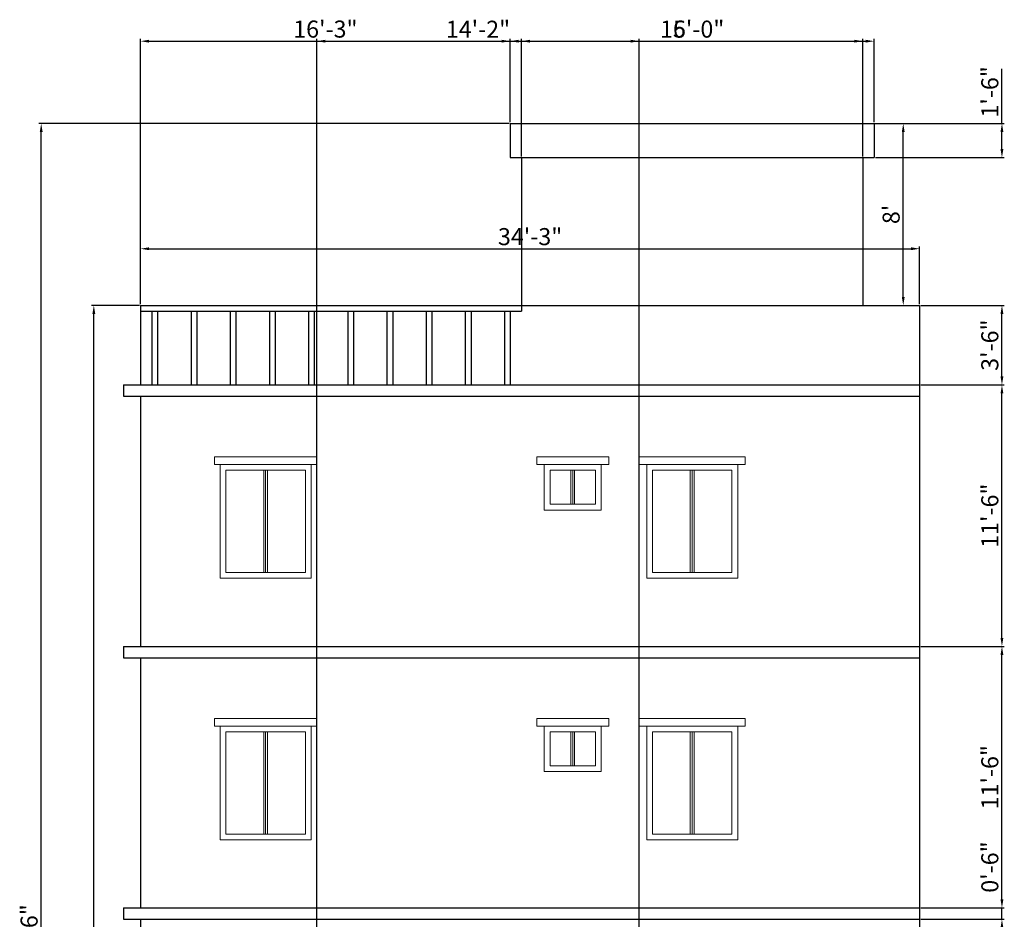
# Model space of a CAD drawing. Units: inches. Extents: x 1692 to 2762, y 798 to 1757.
# Tile 2 of 4: x 1692 to 2211, y 1282 to 1757. Entities that reach past the tile are written whole.
import ezdxf

# ---------------------------------------------------------------- set-up
doc = ezdxf.new("R2010")
doc.units = ezdxf.units.IN
for name, color, linetype, lineweight in [('A-ANNO-DIMS', 2, 'Continuous', 18), ('A-ELEV', 7, 'Continuous', 25), ('A-GLAZ', 4, 'Continuous', 18)]:
    doc.layers.add(name, color=color, linetype=linetype, lineweight=lineweight)
doc.styles.get("Standard").update_dxf_attribs({"font": 'arial.ttf'})
doc.dimstyles.new('ISO-25', dxfattribs={"dimtxt": 9, "dimasz": 4.5, "dimexe": 1.25, "dimexo": 0.625, "dimtad": 1, "dimdec": 0, "dimlunit": 3, "dimtxsty": 'Standard', "dimcen": 2.5, "dimadec": 0, "dimazin": 0, "dimtfac": 1, "dimtdec": 0, "dimtmove": 0, "dimatfit": 3, "dimfxl": 1, "dimarcsym": 0})

# ---------------------------------------------------------------- blocks, each defined once
blk = doc.blocks.new('*D12')
at = {"layer": 'A-ANNO-DIMS', "color": 0, "lineweight": -2, "transparency": 16777216}
for p, q in [((1755.16, 1606.43), (1729.9, 1606.43)), ((1731.15, 848.93), (1731.15, 1601.93)), ((1755.16, 844.43), (1729.9, 844.43))]:
    blk.add_line(p, q, dxfattribs=at)
at = {"layer": 'A-ANNO-DIMS', "color": 0, "lineweight": 0, "transparency": 16777216}
for points in [[(1730.4, 1601.93), (1731.9, 1601.93), (1731.15, 1606.43)], [(1730.4, 848.93), (1731.9, 848.93), (1731.15, 844.43)]]:
    blk.add_solid(points, dxfattribs=at)
at = {"layer": 'Defpoints', "color": 0, "lineweight": 0, "transparency": 16777216}
for p in [(1731.15, 1606.43), (1755.78, 1606.43), (1755.78, 844.43)]:
    blk.add_point(p, dxfattribs=at)
at = {"layer": 'A-ANNO-DIMS', "color": 0, "transparency": 16777216, "insert": (1725.92, 1225.43), "char_height": 9, "attachment_point": 5, "rotation": 90}
blk.add_mtext('63\'-6"', dxfattribs=at)
blk = doc.blocks.new('*D13')
at = {"layer": 'A-ANNO-DIMS', "color": 0, "lineweight": -2, "transparency": 16777216}
for p, q in [((1755.78, 1607.06), (1755.78, 1637.56)), ((1760.28, 1636.31), (2162.28, 1636.31)), ((2166.78, 1607.06), (2166.78, 1637.56))]:
    blk.add_line(p, q, dxfattribs=at)
at = {"layer": 'A-ANNO-DIMS', "color": 0, "lineweight": 0, "transparency": 16777216}
for points in [[(1760.28, 1637.06), (1760.28, 1635.56), (1755.78, 1636.31)], [(2162.28, 1637.06), (2162.28, 1635.56), (2166.78, 1636.31)]]:
    blk.add_solid(points, dxfattribs=at)
at = {"layer": 'Defpoints', "color": 0, "lineweight": 0, "transparency": 16777216}
for p in [(2166.78, 1636.31), (1755.78, 1606.43), (2166.78, 1606.43)]:
    blk.add_point(p, dxfattribs=at)
at = {"layer": 'A-ANNO-DIMS', "color": 0, "transparency": 16777216, "insert": (1961.28, 1641.54), "char_height": 9, "attachment_point": 5}
blk.add_mtext('34\'-3"', dxfattribs=at)
blk = doc.blocks.new('*D14')
at = {"layer": 'A-ANNO-DIMS', "color": 0, "lineweight": -2, "transparency": 16777216}
for p, q in [((2137.41, 1702.43), (2159.37, 1702.43)), ((2158.12, 1610.93), (2158.12, 1697.93)), ((2137.41, 1606.43), (2159.37, 1606.43))]:
    blk.add_line(p, q, dxfattribs=at)
at = {"layer": 'A-ANNO-DIMS', "color": 0, "lineweight": 0, "transparency": 16777216}
for points in [[(2157.37, 1697.93), (2158.87, 1697.93), (2158.12, 1702.43)], [(2157.37, 1610.93), (2158.87, 1610.93), (2158.12, 1606.43)]]:
    blk.add_solid(points, dxfattribs=at)
at = {"layer": 'Defpoints', "color": 0, "lineweight": 0, "transparency": 16777216}
for p in [(2136.78, 1702.43), (2158.12, 1702.43), (2136.78, 1606.43)]:
    blk.add_point(p, dxfattribs=at)
at = {"layer": 'A-ANNO-DIMS', "color": 0, "transparency": 16777216, "insert": (2152.9, 1654.43), "char_height": 9, "attachment_point": 5, "rotation": 90}
blk.add_mtext("8'", dxfattribs=at)
blk = doc.blocks.new('WIN-ELEV-L')
for p, q in [((1794.78, 974.43), (1848.78, 974.43)), ((1794.78, 974.43), (1794.78, 970.43)), ((1797.78, 974.43), (1794.78, 974.43)), ((1845.78, 974.43), (1848.78, 974.43)), ((1848.78, 974.43), (1848.78, 970.43)), ((1794.78, 970.43), (1848.78, 970.43)), ((1797.78, 970.43), (1797.78, 910.43)), ((1800.78, 967.43), (1842.78, 967.43)), ((1800.78, 967.43), (1800.78, 913.43)), ((1820.78, 967.43), (1820.78, 913.43)), ((1821.78, 967.43), (1821.78, 913.43)), ((1822.78, 967.43), (1822.78, 913.43)), ((1842.78, 967.43), (1842.78, 913.43)), ((1845.78, 970.43), (1845.78, 910.43)), ((1797.78, 910.43), (1845.78, 910.43)), ((1797.78, 910.43), (1845.78, 910.43)), ((1800.78, 913.43), (1842.78, 913.43))]:
    blk.add_line(p, q)
blk = doc.blocks.new('WIN-ELEV-R')
for p, q in [((2018.78, 1112.43), (2074.78, 1112.43)), ((2018.78, 1112.43), (2018.78, 1108.43)), ((2074.78, 1112.43), (2074.78, 1108.43)), ((2018.78, 1108.43), (2074.78, 1108.43)), ((2022.78, 1108.43), (2022.78, 1048.43)), ((2070.78, 1108.43), (2070.78, 1048.43)), ((2025.78, 1105.43), (2067.78, 1105.43)), ((2025.78, 1105.43), (2025.78, 1051.43)), ((2045.78, 1105.43), (2045.78, 1051.43)), ((2046.78, 1105.43), (2046.78, 1051.43)), ((2047.78, 1105.43), (2047.78, 1051.43)), ((2067.78, 1105.43), (2067.78, 1051.43)), ((2025.78, 1051.43), (2067.78, 1051.43)), ((2022.78, 1048.43), (2070.78, 1048.43))]:
    blk.add_line(p, q)
blk = doc.blocks.new('WIN-ELEV-S')
for p, q in [((1964.78, 974.43), (2002.78, 974.43)), ((1964.78, 974.43), (1964.78, 970.43)), ((2002.78, 974.43), (2002.78, 970.43)), ((1964.78, 970.43), (2002.78, 970.43)), ((1968.78, 970.43), (1968.78, 946.43)), ((1971.78, 967.43), (1995.78, 967.43)), ((1971.78, 967.43), (1971.78, 949.43)), ((1982.78, 967.43), (1982.78, 949.43)), ((1983.78, 967.43), (1983.78, 949.43)), ((1984.78, 967.43), (1984.78, 949.43)), ((1995.78, 967.43), (1995.78, 949.43)), ((1998.78, 970.43), (1998.78, 946.43)), ((1968.78, 946.43), (1998.78, 946.43)), ((1971.78, 949.43), (1995.78, 949.43))]:
    blk.add_line(p, q)
blk = doc.blocks.new('*D24')
at = {"layer": 'A-ANNO-DIMS', "color": 0, "lineweight": -2, "transparency": 16777216}
for p, q in [((1950.16, 1702.43), (1702.13, 1702.43)), ((1703.38, 848.93), (1703.38, 1697.93)), ((1746.16, 844.43), (1702.13, 844.43))]:
    blk.add_line(p, q, dxfattribs=at)
at = {"layer": 'A-ANNO-DIMS', "color": 0, "lineweight": 0, "transparency": 16777216}
for points in [[(1702.63, 1697.93), (1704.13, 1697.93), (1703.38, 1702.43)], [(1702.63, 848.93), (1704.13, 848.93), (1703.38, 844.43)]]:
    blk.add_solid(points, dxfattribs=at)
at = {"layer": 'Defpoints', "color": 0, "lineweight": 0, "transparency": 16777216}
for p in [(1703.38, 1702.43), (1950.78, 1702.43), (1746.78, 844.43)]:
    blk.add_point(p, dxfattribs=at)
at = {"layer": 'A-ANNO-DIMS', "color": 0, "transparency": 16777216, "insert": (1698.16, 1273.43), "char_height": 9, "attachment_point": 5, "rotation": 90}
blk.add_mtext('71\'-6"', dxfattribs=at)
blk = doc.blocks.new('*D34')
at = {"layer": 'A-ANNO-DIMS', "color": 0, "lineweight": -2, "transparency": 16777216}
for p, q in [((2210.18, 1292.93), (2210.18, 1322.61)), ((2167.41, 1288.43), (2211.43, 1288.43)), ((2210.18, 1282.43), (2210.18, 1288.43)), ((2167.41, 1282.43), (2211.43, 1282.43)), ((2210.18, 1277.93), (2210.18, 1273.43))]:
    blk.add_line(p, q, dxfattribs=at)
at = {"layer": 'A-ANNO-DIMS', "color": 0, "lineweight": 0, "transparency": 16777216}
for points in [[(2209.43, 1292.93), (2210.93, 1292.93), (2210.18, 1288.43)], [(2209.43, 1277.93), (2210.93, 1277.93), (2210.18, 1282.43)]]:
    blk.add_solid(points, dxfattribs=at)
at = {"layer": 'Defpoints', "color": 0, "lineweight": 0, "transparency": 16777216}
for p in [(2166.78, 1288.43), (2210.18, 1288.43), (2166.78, 1282.43)]:
    blk.add_point(p, dxfattribs=at)
at = {"layer": 'A-ANNO-DIMS', "color": 0, "transparency": 16777216, "insert": (2204.96, 1310.02), "char_height": 9, "attachment_point": 5, "rotation": 90}
blk.add_mtext('0\'-6"', dxfattribs=at)
blk = doc.blocks.new('*D35')
at = {"layer": 'A-ANNO-DIMS', "color": 0, "lineweight": -2, "transparency": 16777216}
for p, q in [((2167.41, 1426.43), (2211.43, 1426.43)), ((2210.18, 1292.93), (2210.18, 1421.93)), ((2167.41, 1288.43), (2211.43, 1288.43))]:
    blk.add_line(p, q, dxfattribs=at)
at = {"layer": 'A-ANNO-DIMS', "color": 0, "lineweight": 0, "transparency": 16777216}
for points in [[(2209.43, 1421.93), (2210.93, 1421.93), (2210.18, 1426.43)], [(2209.43, 1292.93), (2210.93, 1292.93), (2210.18, 1288.43)]]:
    blk.add_solid(points, dxfattribs=at)
at = {"layer": 'Defpoints', "color": 0, "lineweight": 0, "transparency": 16777216}
for p in [(2166.78, 1426.43), (2210.18, 1426.43), (2166.78, 1288.43)]:
    blk.add_point(p, dxfattribs=at)
at = {"layer": 'A-ANNO-DIMS', "color": 0, "transparency": 16777216, "insert": (2204.96, 1357.43), "char_height": 9, "attachment_point": 5, "rotation": 90}
blk.add_mtext('11\'-6"', dxfattribs=at)
blk = doc.blocks.new('*D36')
at = {"layer": 'A-ANNO-DIMS', "color": 0, "lineweight": -2, "transparency": 16777216}
for p, q in [((2167.41, 1564.43), (2211.43, 1564.43)), ((2210.18, 1430.93), (2210.18, 1559.93)), ((2167.41, 1426.43), (2211.43, 1426.43))]:
    blk.add_line(p, q, dxfattribs=at)
at = {"layer": 'A-ANNO-DIMS', "color": 0, "lineweight": 0, "transparency": 16777216}
for points in [[(2209.43, 1559.93), (2210.93, 1559.93), (2210.18, 1564.43)], [(2209.43, 1430.93), (2210.93, 1430.93), (2210.18, 1426.43)]]:
    blk.add_solid(points, dxfattribs=at)
at = {"layer": 'Defpoints', "color": 0, "lineweight": 0, "transparency": 16777216}
for p in [(2166.78, 1564.43), (2210.18, 1564.43), (2166.78, 1426.43)]:
    blk.add_point(p, dxfattribs=at)
at = {"layer": 'A-ANNO-DIMS', "color": 0, "transparency": 16777216, "insert": (2204.96, 1495.43), "char_height": 9, "attachment_point": 5, "rotation": 90}
blk.add_mtext('11\'-6"', dxfattribs=at)
blk = doc.blocks.new('*D37')
at = {"layer": 'A-ANNO-DIMS', "color": 0, "lineweight": -2, "transparency": 16777216}
for p, q in [((2167.41, 1606.43), (2211.43, 1606.43)), ((2210.18, 1568.93), (2210.18, 1601.93)), ((2167.41, 1564.43), (2211.43, 1564.43))]:
    blk.add_line(p, q, dxfattribs=at)
at = {"layer": 'A-ANNO-DIMS', "color": 0, "lineweight": 0, "transparency": 16777216}
for points in [[(2209.43, 1601.93), (2210.93, 1601.93), (2210.18, 1606.43)], [(2209.43, 1568.93), (2210.93, 1568.93), (2210.18, 1564.43)]]:
    blk.add_solid(points, dxfattribs=at)
at = {"layer": 'Defpoints', "color": 0, "lineweight": 0, "transparency": 16777216}
for p in [(2166.78, 1606.43), (2210.18, 1606.43), (2166.78, 1564.43)]:
    blk.add_point(p, dxfattribs=at)
at = {"layer": 'A-ANNO-DIMS', "color": 0, "transparency": 16777216, "insert": (2204.96, 1585.43), "char_height": 9, "attachment_point": 5, "rotation": 90}
blk.add_mtext('3\'-6"', dxfattribs=at)
blk = doc.blocks.new('*D38')
at = {"layer": 'A-ANNO-DIMS', "color": 0, "lineweight": -2, "transparency": 16777216}
for p, q in [((2210.18, 1702.43), (2210.18, 1731.26)), ((2143.41, 1702.43), (2211.43, 1702.43)), ((2210.18, 1688.93), (2210.18, 1697.93)), ((2143.41, 1684.43), (2211.43, 1684.43))]:
    blk.add_line(p, q, dxfattribs=at)
at = {"layer": 'A-ANNO-DIMS', "color": 0, "lineweight": 0, "transparency": 16777216}
for points in [[(2209.43, 1697.93), (2210.93, 1697.93), (2210.18, 1702.43)], [(2209.43, 1688.93), (2210.93, 1688.93), (2210.18, 1684.43)]]:
    blk.add_solid(points, dxfattribs=at)
at = {"layer": 'Defpoints', "color": 0, "lineweight": 0, "transparency": 16777216}
for p in [(2142.78, 1702.43), (2210.18, 1702.43), (2142.78, 1684.43)]:
    blk.add_point(p, dxfattribs=at)
at = {"layer": 'A-ANNO-DIMS', "color": 0, "transparency": 16777216, "insert": (2204.96, 1719.1), "char_height": 9, "attachment_point": 5, "rotation": 90}
blk.add_mtext('1\'-6"', dxfattribs=at)
blk = doc.blocks.new('*D47')
at = {"layer": 'A-ANNO-DIMS', "color": 0, "lineweight": -2, "transparency": 16777216}
for p, q in [((1848.78, 1113.06), (1848.78, 1747.08)), ((1853.28, 1745.83), (2014.28, 1745.83)), ((2018.78, 1113.06), (2018.78, 1747.08))]:
    blk.add_line(p, q, dxfattribs=at)
at = {"layer": 'A-ANNO-DIMS', "color": 0, "lineweight": 0, "transparency": 16777216}
for points in [[(1853.28, 1746.58), (1853.28, 1745.08), (1848.78, 1745.83)], [(2014.28, 1746.58), (2014.28, 1745.08), (2018.78, 1745.83)]]:
    blk.add_solid(points, dxfattribs=at)
at = {"layer": 'Defpoints', "color": 0, "lineweight": 0, "transparency": 16777216}
for p in [(2018.78, 1745.83), (1848.78, 1112.43), (2018.78, 1112.43)]:
    blk.add_point(p, dxfattribs=at)
at = {"layer": 'A-ANNO-DIMS', "color": 0, "transparency": 16777216, "insert": (1933.78, 1750.98), "char_height": 9, "attachment_point": 5}
blk.add_mtext('14\'-2"', dxfattribs=at)
blk = doc.blocks.new('*D48')
at = {"layer": 'A-ANNO-DIMS', "color": 0, "lineweight": -2, "transparency": 16777216}
for p, q in [((1755.78, 1607.06), (1755.78, 1747.08)), ((1760.28, 1745.83), (1946.28, 1745.83)), ((1950.78, 1703.06), (1950.78, 1747.08))]:
    blk.add_line(p, q, dxfattribs=at)
at = {"layer": 'A-ANNO-DIMS', "color": 0, "lineweight": 0, "transparency": 16777216}
for points in [[(1760.28, 1746.58), (1760.28, 1745.08), (1755.78, 1745.83)], [(1946.28, 1746.58), (1946.28, 1745.08), (1950.78, 1745.83)]]:
    blk.add_solid(points, dxfattribs=at)
at = {"layer": 'Defpoints', "color": 0, "lineweight": 0, "transparency": 16777216}
for p in [(1950.78, 1745.83), (1950.78, 1702.43), (1755.78, 1606.43)]:
    blk.add_point(p, dxfattribs=at)
at = {"layer": 'A-ANNO-DIMS', "color": 0, "transparency": 16777216, "insert": (1853.28, 1751.06), "char_height": 9, "attachment_point": 5}
blk.add_mtext('16\'-3"', dxfattribs=at)
blk = doc.blocks.new('*D49')
at = {"layer": 'A-ANNO-DIMS', "color": 0, "lineweight": -2, "transparency": 16777216}
for p, q in [((1950.78, 1703.06), (1950.78, 1747.08)), ((1955.28, 1745.83), (2138.28, 1745.83)), ((2142.78, 1703.06), (2142.78, 1747.08))]:
    blk.add_line(p, q, dxfattribs=at)
at = {"layer": 'A-ANNO-DIMS', "color": 0, "lineweight": 0, "transparency": 16777216}
for points in [[(1955.28, 1746.58), (1955.28, 1745.08), (1950.78, 1745.83)], [(2138.28, 1746.58), (2138.28, 1745.08), (2142.78, 1745.83)]]:
    blk.add_solid(points, dxfattribs=at)
at = {"layer": 'Defpoints', "color": 0, "lineweight": 0, "transparency": 16777216}
for p in [(2142.78, 1745.83), (1950.78, 1702.43), (2142.78, 1702.43)]:
    blk.add_point(p, dxfattribs=at)
at = {"layer": 'A-ANNO-DIMS', "color": 0, "transparency": 16777216, "insert": (2046.78, 1751.05), "char_height": 9, "attachment_point": 5}
blk.add_mtext('16\'-0"', dxfattribs=at)
blk = doc.blocks.new('*D50')
at = {"layer": 'A-ANNO-DIMS', "color": 0, "lineweight": -2, "transparency": 16777216}
for p, q in [((1956.78, 1685.06), (1956.78, 1747.08)), ((1961.28, 1745.83), (2132.28, 1745.83)), ((2136.78, 1685.06), (2136.78, 1747.08))]:
    blk.add_line(p, q, dxfattribs=at)
at = {"layer": 'A-ANNO-DIMS', "color": 0, "lineweight": 0, "transparency": 16777216}
for points in [[(1961.28, 1746.58), (1961.28, 1745.08), (1956.78, 1745.83)], [(2132.28, 1746.58), (2132.28, 1745.08), (2136.78, 1745.83)]]:
    blk.add_solid(points, dxfattribs=at)
at = {"layer": 'Defpoints', "color": 0, "lineweight": 0, "transparency": 16777216}
for p in [(2136.78, 1745.83), (1956.78, 1684.43), (2136.78, 1684.43)]:
    blk.add_point(p, dxfattribs=at)
at = {"layer": 'A-ANNO-DIMS', "color": 0, "transparency": 16777216, "insert": (2046.78, 1751.05), "char_height": 9, "attachment_point": 5}
blk.add_mtext('15\'-0"', dxfattribs=at)

msp = doc.modelspace()

# ---------------------------------------------------------------- linework, layer by layer
at = {"layer": 'A-ELEV'}
for p, q in [((1950.78, 1702.43), (2142.78, 1702.43)), ((1950.78, 1702.43), (1950.78, 1684.43)), ((2142.78, 1702.43), (2142.78, 1684.43)), ((1950.78, 1684.43), (2142.78, 1684.43)), ((1956.78, 1684.43), (1956.78, 1603.43)), ((2136.78, 1684.43), (2136.78, 1606.43)), ((1755.78, 1606.43), (2166.78, 1606.43)), ((1755.78, 1606.43), (1755.78, 1564.43)), ((2166.78, 1606.43), (2166.78, 1006.43)), ((1755.78, 1603.43), (1956.78, 1603.43)), ((1761.77, 1603.43), (1761.77, 1564.43)), ((1764.77, 1603.43), (1764.77, 1564.43)), ((1782.44, 1603.43), (1782.44, 1564.43)), ((1785.44, 1603.43), (1785.44, 1564.43)), ((1803.1, 1603.43), (1803.1, 1564.43)), ((1806.1, 1603.43), (1806.1, 1564.43)), ((1823.77, 1603.43), (1823.77, 1564.43)), ((1826.77, 1603.43), (1826.77, 1564.43)), ((1844.44, 1603.43), (1844.44, 1564.43)), ((1847.44, 1603.43), (1847.44, 1564.43)), ((1865.11, 1603.43), (1865.11, 1564.43)), ((1868.11, 1603.43), (1868.11, 1564.43)), ((1885.78, 1603.43), (1885.78, 1564.43)), ((1888.78, 1603.43), (1888.78, 1564.43)), ((1906.44, 1603.43), (1906.44, 1564.43)), ((1909.44, 1603.43), (1909.44, 1564.43)), ((1927.11, 1603.43), (1927.11, 1564.43)), ((1930.11, 1603.43), (1930.11, 1564.43)), ((1947.78, 1603.43), (1947.78, 1564.43)), ((1950.78, 1603.43), (1950.78, 1564.43)), ((1746.78, 1564.43), (2166.78, 1564.43)), ((1746.78, 1564.43), (1746.78, 1558.43)), ((1746.78, 1558.43), (2166.78, 1558.43)), ((1755.78, 1558.43), (1755.78, 1426.43)), ((1746.78, 1426.43), (2166.78, 1426.43)), ((1746.78, 1426.43), (1746.78, 1420.43)), ((1746.78, 1420.43), (2166.78, 1420.43)), ((1755.78, 1420.43), (1755.78, 1288.43)), ((1746.78, 1288.43), (2166.78, 1288.43)), ((1746.78, 1288.43), (1746.78, 1282.43)), ((1746.78, 1282.43), (2166.78, 1282.43)), ((1755.78, 1282.43), (1755.78, 1150.43))]:
    msp.add_line(p, q, dxfattribs=at)

# ---------------------------------------------------------------- block references
at = {"layer": 'A-GLAZ'}
for name, p in [('WIN-ELEV-L', (0, 552)), ('WIN-ELEV-S', (0, 552)), ('WIN-ELEV-R', (0, 414)), ('WIN-ELEV-L', (0, 414)), ('WIN-ELEV-S', (0, 414)), ('WIN-ELEV-R', (0, 276))]:
    msp.add_blockref(name, p, dxfattribs=at)

# ---------------------------------------------------------------- dimensions: what is measured, and where the dimension line sits
at = {"layer": 'A-ANNO-DIMS'}
for base, p1, p2, override, picture, middle in [((1950.78, 1745.83), (1755.78, 1606.43), (1950.78, 1702.43), {"dimdec": 1, "dimlfac": 1, "dimrnd": 0, "dimzin": 1, "dimdsep": 46, "dimlunit": 4, "dimfrac": 2}, '*D48', (1853.28, 1751.06)), ((2018.78, 1745.83), (1848.78, 1112.43), (2018.78, 1112.43), {"dimdec": 1, "dimlfac": 1, "dimrnd": 0, "dimzin": 1, "dimdsep": 46, "dimlunit": 4, "dimfrac": 2}, '*D47', (1933.78, 1750.98)), ((2142.78, 1745.83), (1950.78, 1702.43), (2142.78, 1702.43), {"dimdec": 1, "dimlfac": 1, "dimrnd": 0, "dimzin": 1, "dimdsep": 46, "dimlunit": 4, "dimfrac": 2}, '*D49', (2046.78, 1751.05)), ((2136.78, 1745.83), (1956.78, 1684.43), (2136.78, 1684.43), {"dimdec": 1, "dimlfac": 1, "dimrnd": 0, "dimzin": 1, "dimdsep": 46, "dimlunit": 4, "dimfrac": 2}, '*D50', (2046.78, 1751.05)), ((2166.78, 1636.31), (1755.78, 1606.43), (2166.78, 1606.43), {"dimclrd": 0, "dimclre": 0, "dimclrt": 0}, '*D13', (1961.28, 1641.54))]:
    dim = msp.add_linear_dim(base=base, p1=p1, p2=p2, dimstyle='ISO-25', override=override, dxfattribs=at)
    dim.commit()
    dim.dimension.update_dxf_attribs({"geometry": picture, "text_midpoint": middle})
for base, p1, p2, override, picture, middle in [((2210.18, 1702.43), (2142.78, 1684.43), (2142.78, 1702.43), {"dimdec": 1, "dimlfac": 1, "dimrnd": 0, "dimzin": 1, "dimdsep": 46, "dimlunit": 4, "dimfrac": 2}, '*D38', (2204.96, 1719.1)), ((1703.38, 1702.43), (1746.78, 844.43), (1950.78, 1702.43), {"dimdec": 1, "dimlfac": 1, "dimrnd": 0, "dimzin": 1, "dimdsep": 46, "dimlunit": 4, "dimfrac": 2}, '*D24', (1698.16, 1273.43)), ((2158.12, 1702.43), (2136.78, 1606.43), (2136.78, 1702.43), {"dimclrd": 0, "dimclre": 0, "dimclrt": 0}, '*D14', (2152.9, 1654.43)), ((1731.15, 1606.43), (1755.78, 844.43), (1755.78, 1606.43), {"dimclrd": 0, "dimclre": 0, "dimclrt": 0}, '*D12', (1725.92, 1225.43)), ((2210.18, 1606.43), (2166.78, 1564.43), (2166.78, 1606.43), {"dimdec": 1, "dimlfac": 1, "dimrnd": 0, "dimzin": 1, "dimdsep": 46, "dimlunit": 4, "dimfrac": 2}, '*D37', (2204.96, 1585.43)), ((2210.18, 1564.43), (2166.78, 1426.43), (2166.78, 1564.43), {"dimdec": 1, "dimlfac": 1, "dimrnd": 0, "dimzin": 1, "dimdsep": 46, "dimlunit": 4, "dimfrac": 2}, '*D36', (2204.96, 1495.43)), ((2210.18, 1426.43), (2166.78, 1288.43), (2166.78, 1426.43), {"dimdec": 1, "dimlfac": 1, "dimrnd": 0, "dimzin": 1, "dimdsep": 46, "dimlunit": 4, "dimfrac": 2}, '*D35', (2204.96, 1357.43)), ((2210.18, 1288.43), (2166.78, 1282.43), (2166.78, 1288.43), {"dimdec": 1, "dimlfac": 1, "dimrnd": 0, "dimzin": 1, "dimdsep": 46, "dimlunit": 4, "dimfrac": 2}, '*D34', (2204.96, 1310.02))]:
    dim = msp.add_linear_dim(base=base, p1=p1, p2=p2, angle=90, dimstyle='ISO-25', override=override, dxfattribs=at)
    dim.commit()
    dim.dimension.update_dxf_attribs({"geometry": picture, "text_midpoint": middle})

doc.saveas('drawing.dxf')
